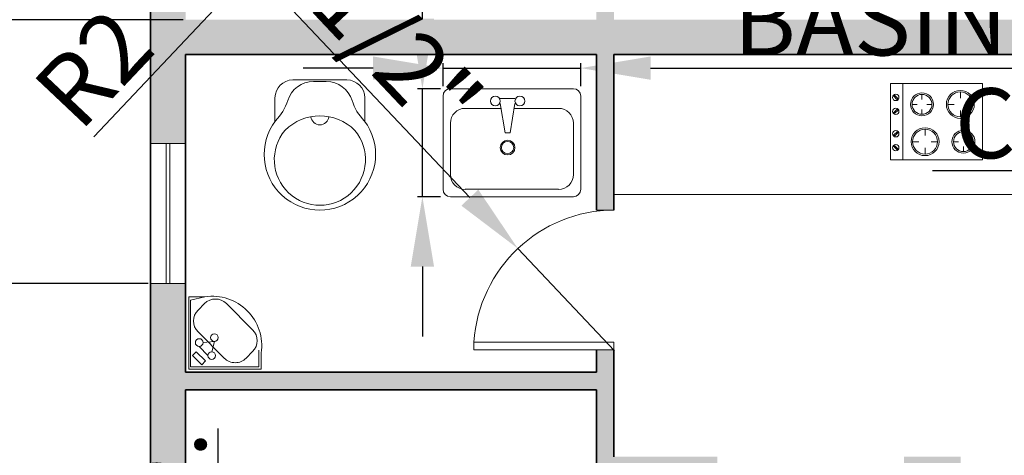
# Model space of a CAD drawing. Units: inches. Extents: x 2043 to 3177, y 1429 to 2563.
# Tile 4 of 14: x 2200 to 2453, y 1840 to 1952. Entities that reach past the tile are written whole.
import ezdxf

# ---------------------------------------------------------------- set-up
doc = ezdxf.new("R2010")
doc.units = ezdxf.units.IN
for name, color, linetype, lineweight in [('A-ANNO-DIMS', 2, 'Continuous', 13), ('A-DOOR', 3, 'Continuous', 18), ('A-EQPM', 8, 'Continuous', 18), ('A-FLOR-CASE', 8, 'Continuous', 18), ('A-FLOR-FIXT', 8, 'Continuous', 18), ('A-GLAZ', 4, 'Continuous', 18), ('A-WALL', 7, 'Continuous', 35)]:
    doc.layers.add(name, color=color, linetype=linetype, lineweight=lineweight)
doc.layers.add('A-WALL-PATT', color=251, linetype='Continuous', lineweight=13, true_color=0x636466)
doc.styles.add('DIM_FONT', font='TXT.shx', dxfattribs={"width": 0.8})
doc.styles.get("Standard").update_dxf_attribs({"font": 'arial.ttf'})
doc.dimstyles.new('ISO-25', dxfattribs={"dimtxt": 18, "dimasz": 18, "dimexe": 1.25, "dimexo": 0.625, "dimtad": 1, "dimlunit": 3, "dimtxsty": 'Standard', "dimcen": 2.5, "dimadec": 0, "dimazin": 0, "dimtfac": 1, "dimtmove": 0, "dimatfit": 3, "dimfxl": 1, "dimarcsym": 0})

# ---------------------------------------------------------------- blocks, each defined once
blk = doc.blocks.new('A$C6EF51710')
at = {"linetype": 'ByBlock'}
for p, q in [((0.0508, 0.2843), (0.1169, 0.2843)), ((0, 0.0811), (0, 0.2335)), ((0.0041, 0.1392), (0.0041, 0.1755)), ((0.1169, 0.0303), (0.0508, 0.0303))]:
    blk.add_line(p, q, dxfattribs=at)
for centre, radius, start, end in [((0.2107, 0.1573), 0.1576, 232.8984, 127.1016), ((0.0508, 0.2335), 0.0508, 90, 180), ((0.0168, 0.3818), 0.1397, 287.1046, 315), ((0.2254, 0.1573), 0.1289, 230.0084, 129.9916), ((0.2413, 0.1573), 0.1397, 135, 225), ((0.0803, 0.1755), 0.0762, 107.1046, 180), ((0.1016, 0.1573), 0.0254, 275.2159, 84.7841), ((0.0803, 0.1392), 0.0762, 180, 252.8954), ((0.0508, 0.0811), 0.0508, 180, 270), ((0.0168, -0.0672), 0.1397, 45, 72.8954)]:
    blk.add_arc(centre, radius, start, end, dxfattribs=at)
blk = doc.blocks.new('A$C03A44EBA')
at = {"rotation": 270}
blk.add_blockref('A$C6EF51710', (0.0003, 0.3683), dxfattribs=at)
blk = doc.blocks.new('A$C564A496C')
at = {"linetype": 'ByBlock'}
for p, q in [((0, 419.3), (0, 30.7)), ((543.2, 450), (30.7, 450)), ((573.8, 30.7), (573.8, 419.3)), ((238.5, 409.1), (299.8, 409.1)), ((238.5, 388.6), (258.9, 265.9)), ((279.4, 265.9), (299.8, 388.6)), ((92, 368.2), (243.6, 368.2)), ((294.7, 368.2), (481.8, 368.2)), ((30.7, 92), (30.7, 306.8)), ((543.2, 306.8), (543.2, 92)), ((258.9, 265.9), (279.4, 265.9)), ((30.7, 0), (543.2, 0)), ((481.8, 30.7), (92, 30.7))]:
    blk.add_line(p, q, dxfattribs=at)
for centre, radius in [((218, 398.9), 20.5), ((320.3, 398.9), 20.5), ((269.1, 204.5), 30.7), ((269.1, 204.5), 25.7)]:
    blk.add_circle(centre, radius, dxfattribs=at)
for centre, radius, start, end in [((30.7, 419.3), 30.7, 90, 180), ((543.2, 419.3), 30.7, 0, 90), ((92, 306.8), 61.4, 90, 180), ((481.8, 306.8), 61.4, 0, 90), ((92, 92), 61.4, 180, 270), ((481.8, 92), 61.4, 270, 0), ((30.7, 30.7), 30.7, 180, 270), ((543.2, 30.7), 30.7, 270, 0)]:
    blk.add_arc(centre, radius, start, end, dxfattribs=at)
at = {"style": 'DIM_FONT', "width": 0.8, "flags": 9}
for tag in ['YSIZE', 'XSIZE']:
    blk.add_attdef(tag, (269.1, 450), '', height=0.5, rotation=270, dxfattribs=at)
blk = doc.blocks.new('A$C017A17F4')
for p, q in [((0.45, 0.45), (0, 0.45)), ((0, 0.45), (0, 0.35)), ((0.45, 0), (0.45, 0.45)), ((0.0533, 0.3414), (0.094, 0.3821)), ((0.2297, 0.3821), (0.3933, 0.2185)), ((0.3467, 0.3997), (0.3704, 0.4234)), ((0.4041, 0.3423), (0.3467, 0.3997)), ((0.3704, 0.4234), (0.4278, 0.366)), ((0.4278, 0.366), (0.4041, 0.3423)), ((0.2168, 0.0421), (0.0533, 0.2056)), ((0.3933, 0.0827), (0.3526, 0.0421)), ((0.35, 0), (0.45, 0))]:
    blk.add_line(p, q)
at = {"ltscale": 10}
for p, q in [((0.4392, 0.4359), (0.0144, 0.4359)), ((0.0144, 0.4359), (0.0144, 0.3323)), ((0.4392, 0.4359), (0.4392, 0.0216)), ((0.3078, 0.342), (0.2911, 0.2778)), ((0.3317, 0.3659), (0.3861, 0.3086)), ((0.3622, 0.2847), (0.2911, 0.2778)), ((0.4392, 0.0216), (0.35, 0))]:
    blk.add_line(p, q, dxfattribs=at)
for centre in [(0.3078, 0.3659), (0.3861, 0.2847), (0.2911, 0.2539)]:
    blk.add_circle(centre, 0.0239, dxfattribs=at)
for centre, radius, start, end in [((0.1618, 0.3142), 0.096, 45, 135), ((0.3045, 0.3045), 0.3079, 171.50989, 278.49011), ((0.1212, 0.2735), 0.096, 135, 225), ((0.3254, 0.1506), 0.096, 315, 45), ((0.2847, 0.11), 0.096, 225, 315)]:
    blk.add_arc(centre, radius, start, end)
blk = doc.blocks.new('*D25')
at = {"layer": 'A-ANNO-DIMS', "color": 0, "lineweight": -2, "transparency": 16777216}
for p, q in [((2233.12, 1884.52), (2167.18, 1884.52)), ((2168.43, 1652.39), (2168.43, 1866.52)), ((2233.12, 1634.39), (2167.18, 1634.39))]:
    blk.add_line(p, q, dxfattribs=at)
at = {"layer": 'A-ANNO-DIMS', "color": 0, "transparency": 16777216}
for points in [[(2165.43, 1866.52), (2171.43, 1866.52), (2168.43, 1884.52)], [(2165.43, 1652.39), (2171.43, 1652.39), (2168.43, 1634.39)]]:
    blk.add_solid(points, dxfattribs=at)
at = {"layer": 'Defpoints', "color": 0, "transparency": 16777216}
for p in [(2168.43, 1884.52), (2233.74, 1884.52), (2233.74, 1634.39)]:
    blk.add_point(p, dxfattribs=at)
at = {"layer": 'A-ANNO-DIMS', "color": 0, "transparency": 16777216, "insert": (2158.61, 1759.46), "char_height": 18, "attachment_point": 5, "rotation": 90}
blk.add_mtext('25\'-0"', dxfattribs=at)
blk = doc.blocks.new('*D26')
at = {"layer": 'A-ANNO-DIMS', "color": 0, "lineweight": -2, "transparency": 16777216}
for p, q in [((2233.12, 2029.27), (2166.79, 2029.27)), ((2168.04, 1902.52), (2168.04, 2011.27)), ((2233.12, 1884.52), (2166.79, 1884.52))]:
    blk.add_line(p, q, dxfattribs=at)
at = {"layer": 'A-ANNO-DIMS', "color": 0, "transparency": 16777216}
for points in [[(2165.04, 2011.27), (2171.04, 2011.27), (2168.04, 2029.27)], [(2165.04, 1902.52), (2171.04, 1902.52), (2168.04, 1884.52)]]:
    blk.add_solid(points, dxfattribs=at)
at = {"layer": 'Defpoints', "color": 0, "transparency": 16777216}
for p in [(2168.04, 2029.27), (2233.74, 2029.27), (2233.74, 1884.52)]:
    blk.add_point(p, dxfattribs=at)
at = {"layer": 'A-ANNO-DIMS', "color": 0, "transparency": 16777216, "insert": (2158.23, 1956.89), "char_height": 18, "attachment_point": 5, "rotation": 90}
blk.add_mtext('19\'-0"', dxfattribs=at)
blk = doc.blocks.new('*D28')
at = {"layer": 'A-ANNO-DIMS', "color": 0, "lineweight": -2, "transparency": 16777216}
for p, q in [((2233.12, 2261.39), (2064.1, 2261.39)), ((2065.35, 2243.39), (2065.35, 1652.39)), ((2233.12, 1634.39), (2064.1, 1634.39))]:
    blk.add_line(p, q, dxfattribs=at)
at = {"layer": 'A-ANNO-DIMS', "color": 0, "transparency": 16777216}
for points in [[(2062.35, 2243.39), (2068.35, 2243.39), (2065.35, 2261.39)], [(2062.35, 1652.39), (2068.35, 1652.39), (2065.35, 1634.39)]]:
    blk.add_solid(points, dxfattribs=at)
at = {"layer": 'Defpoints', "color": 0, "transparency": 16777216}
for p in [(2233.74, 2261.39), (2065.35, 1634.39), (2233.74, 1634.39)]:
    blk.add_point(p, dxfattribs=at)
at = {"layer": 'A-ANNO-DIMS', "color": 0, "transparency": 16777216, "insert": (2055.54, 1947.89), "char_height": 18, "attachment_point": 5, "rotation": 90}
blk.add_mtext('75\'-0"', dxfattribs=at)
blk = doc.blocks.new('A$C16A60262')
at = {"linetype": 'ByBlock'}
for p, q in [((0, 600), (0, 0)), ((487.7, 600), (0, 600)), ((0, 600), (500, 600)), ((0, 600), (500, 600)), ((500, 600), (500, 0)), ((500, 600), (500, 0)), ((500, 520.4), (0, 520.4)), ((119.4, 455.6), (119.4, 414.9)), ((363.3, 459.6), (363.3, 427.1)), ((298.2, 394.6), (330.7, 394.6)), ((428.3, 394.6), (395.8, 394.6)), ((38.1, 374.3), (78.8, 374.3)), ((119.4, 293), (119.4, 333.7)), ((200.7, 374.3), (160.1, 374.3)), ((363.3, 329.6), (363.3, 362.1)), ((363.3, 225.2), (363.3, 184.6)), ((119.4, 188.6), (119.4, 156.1)), ((282, 143.9), (322.6, 143.9)), ((444.5, 143.9), (403.9, 143.9)), ((54.4, 123.6), (86.9, 123.6)), ((119.4, 58.6), (119.4, 91.1)), ((184.4, 123.6), (151.9, 123.6)), ((363.3, 62.6), (363.3, 103.3)), ((0, 0), (500, 0))]:
    blk.add_line(p, q, dxfattribs=at)
for p, q in [((396.2, 558.5), (417.4, 579.7)), ((417.4, 579.7), (423.1, 574)), ((66.2, 557.5), (87.4, 578.7)), ((71.9, 551.8), (66.2, 557.5)), ((93.1, 573), (71.9, 551.8)), ((87.4, 578.7), (93.1, 573)), ((157.6, 572.5), (163.3, 578.1)), ((178.8, 551.2), (157.6, 572.5)), ((163.3, 578.1), (184.5, 556.9)), ((184.5, 556.9), (178.8, 551.2)), ((305.1, 572.5), (310.8, 578.1)), ((326.3, 551.2), (305.1, 572.5)), ((310.8, 578.1), (332, 556.9)), ((332, 556.9), (326.3, 551.2)), ((401.9, 552.8), (396.2, 558.5)), ((423.1, 574), (401.9, 552.8))]:
    blk.add_line(p, q)
for centre in [(80.1, 565.7), (171.2, 565.7), (317.6, 565.7), (408.7, 565.7)]:
    blk.add_circle(centre, 20.6)
for centre, radius in [((119.4, 374.3), 91.3), ((119.4, 374.3), 81.3), ((363.3, 394.6), 75), ((363.3, 394.6), 65), ((119.4, 123.6), 75), ((363.3, 143.9), 91.3), ((363.3, 143.9), 81.3), ((119.4, 123.6), 65)]:
    blk.add_circle(centre, radius, dxfattribs=at)
blk = doc.blocks.new('GLAZING-36')
for p, q in [((0, 36), (0, 0)), ((1, 36), (1, 0))]:
    blk.add_line(p, q)
blk = doc.blocks.new('*D48')
at = {"layer": 'A-ANNO-DIMS', "color": 0, "lineweight": -2, "transparency": 16777216}
for p, q in [((2251.17, 1717.89), (2251.17, 1847.17)), ((2254.14, 1699.89), (2249.92, 1699.89)), ((2251.17, 1675.89), (2251.17, 1699.89)), ((2254.14, 1675.89), (2249.92, 1675.89)), ((2251.17, 1657.89), (2251.17, 1639.89))]:
    blk.add_line(p, q, dxfattribs=at)
at = {"layer": 'A-ANNO-DIMS', "color": 0, "transparency": 16777216}
for points in [[(2248.17, 1717.89), (2254.17, 1717.89), (2251.17, 1699.89)], [(2248.17, 1657.89), (2254.17, 1657.89), (2251.17, 1675.89)]]:
    blk.add_solid(points, dxfattribs=at)
at = {"layer": 'Defpoints', "color": 0, "transparency": 16777216}
for p in [(2251.17, 1699.89), (2254.77, 1699.89), (2254.77, 1675.89)]:
    blk.add_point(p, dxfattribs=at)
at = {"layer": 'A-ANNO-DIMS', "color": 0, "transparency": 16777216, "insert": (2241.35, 1791.53), "char_height": 18, "attachment_point": 5, "rotation": 90}
blk.add_mtext('2\'-0" TYP.', dxfattribs=at)
blk = doc.blocks.new('*D57')
at = {"layer": 'A-ANNO-DIMS', "color": 0, "lineweight": -2, "transparency": 16777216}
for p, q in [((2291.03, 1939.93), (2273.03, 1939.93)), ((2309.03, 1935.24), (2309.03, 1941.18)), ((2309.03, 1939.93), (2344.46, 1939.93)), ((2344.46, 1935.24), (2344.46, 1941.18)), ((2362.46, 1939.93), (2629.01, 1939.93))]:
    blk.add_line(p, q, dxfattribs=at)
at = {"layer": 'A-ANNO-DIMS', "color": 0, "transparency": 16777216}
for points in [[(2291.03, 1942.93), (2291.03, 1936.93), (2309.03, 1939.93)], [(2362.46, 1942.93), (2362.46, 1936.93), (2344.46, 1939.93)]]:
    blk.add_solid(points, dxfattribs=at)
at = {"layer": 'Defpoints', "color": 0, "transparency": 16777216}
for p in [(2344.46, 1939.93), (2309.03, 1934.62), (2344.46, 1934.62)]:
    blk.add_point(p, dxfattribs=at)
at = {"layer": 'A-ANNO-DIMS', "color": 0, "transparency": 16777216, "insert": (2504.74, 1949.86), "char_height": 18, "attachment_point": 5}
blk.add_mtext('BASIN 2\'-11 1/2" TYP.', dxfattribs=at)
blk = doc.blocks.new('*D58')
at = {"layer": 'A-ANNO-DIMS', "color": 0, "lineweight": -2, "transparency": 16777216}
for p, q in [((2303.72, 1952.62), (2303.72, 2081.89)), ((2308.41, 1934.62), (2302.47, 1934.62)), ((2303.72, 1906.83), (2303.72, 1934.62)), ((2308.41, 1906.83), (2302.47, 1906.83)), ((2303.72, 1888.83), (2303.72, 1870.83))]:
    blk.add_line(p, q, dxfattribs=at)
at = {"layer": 'A-ANNO-DIMS', "color": 0, "transparency": 16777216}
for points in [[(2300.72, 1952.62), (2306.72, 1952.62), (2303.72, 1934.62)], [(2300.72, 1888.83), (2306.72, 1888.83), (2303.72, 1906.83)]]:
    blk.add_solid(points, dxfattribs=at)
at = {"layer": 'Defpoints', "color": 0, "transparency": 16777216}
for p in [(2303.72, 1934.62), (2309.03, 1934.62), (2309.03, 1906.83)]:
    blk.add_point(p, dxfattribs=at)
at = {"layer": 'A-ANNO-DIMS', "color": 0, "transparency": 16777216, "insert": (2294.05, 2026.26), "char_height": 18, "attachment_point": 5, "rotation": 90}
blk.add_mtext('2\'-4" TYP.', dxfattribs=at)
blk = doc.blocks.new('*D61')
at = {"layer": 'A-ANNO-DIMS', "color": 0, "lineweight": -2, "transparency": 16777216}
for p, q in [((2770.39, 1916.38), (2770.39, 1912.21)), ((2794.01, 1916.38), (2794.01, 1912.21)), ((2752.39, 1913.46), (2434.98, 1913.46)), ((2794.01, 1913.46), (2770.39, 1913.46)), ((2812.01, 1913.46), (2830.01, 1913.46))]:
    blk.add_line(p, q, dxfattribs=at)
at = {"layer": 'A-ANNO-DIMS', "color": 0, "transparency": 16777216}
for points in [[(2752.39, 1916.46), (2752.39, 1910.46), (2770.39, 1913.46)], [(2812.01, 1916.46), (2812.01, 1910.46), (2794.01, 1913.46)]]:
    blk.add_solid(points, dxfattribs=at)
at = {"layer": 'Defpoints', "color": 0, "transparency": 16777216}
for p in [(2770.39, 1917.01), (2794.01, 1917.01), (2770.39, 1913.46)]:
    blk.add_point(p, dxfattribs=at)
at = {"layer": 'A-ANNO-DIMS', "color": 0, "transparency": 16777216, "insert": (2584.68, 1923.4), "char_height": 18, "attachment_point": 5}
blk.add_mtext('COOKTOP 1\'-11 1/2" TYP.', dxfattribs=at)
blk = doc.blocks.new('*D74')
at = {"layer": 'A-ANNO-DIMS', "color": 0, "lineweight": -2, "transparency": 16777216}
for p, q in [((2242.12, 1952.39), (2178.39, 1952.39)), ((2179.64, 1652.39), (2179.64, 1934.39)), ((2233.12, 1634.39), (2178.39, 1634.39))]:
    blk.add_line(p, q, dxfattribs=at)
at = {"layer": 'A-ANNO-DIMS', "color": 0, "transparency": 16777216}
for points in [[(2176.64, 1934.39), (2182.64, 1934.39), (2179.64, 1952.39)], [(2176.64, 1652.39), (2182.64, 1652.39), (2179.64, 1634.39)]]:
    blk.add_solid(points, dxfattribs=at)
at = {"layer": 'Defpoints', "color": 0, "transparency": 16777216}
for p in [(2179.64, 1952.39), (2242.74, 1952.39), (2233.74, 1634.39)]:
    blk.add_point(p, dxfattribs=at)
at = {"layer": 'A-ANNO-DIMS', "color": 0, "transparency": 16777216, "insert": (2169.83, 1793.39), "char_height": 18, "attachment_point": 5, "rotation": 90}
blk.add_mtext('26\'-6"', dxfattribs=at)
blk = doc.blocks.new('*D86')
at = {"layer": 'A-ANNO-DIMS', "color": 0, "lineweight": -2, "transparency": 16777216}
for p, q in [((2598.87, 1881.94), (2565.26, 1849.73)), ((2451, 1740.24), (2552.26, 1837.28))]:
    blk.add_line(p, q, dxfattribs=at)
at = {"layer": 'A-ANNO-DIMS', "color": 0, "transparency": 16777216}
blk.add_solid([(2550.18, 1839.44), (2554.34, 1835.11), (2565.26, 1849.73)], dxfattribs=at)
at = {"layer": 'Defpoints', "color": 0, "transparency": 16777216}
for p in [(2598.87, 1881.94), (2565.26, 1849.73)]:
    blk.add_point(p, dxfattribs=at)
at = {"layer": 'A-ANNO-DIMS', "color": 0, "transparency": 16777216, "insert": (2488.26, 1789.71), "char_height": 18, "attachment_point": 5, "rotation": 43.781}
blk.add_mtext('R3\'-10 1/2"', dxfattribs=at)
blk = doc.blocks.new('*D91')
at = {"layer": 'A-ANNO-DIMS', "color": 0, "lineweight": -2, "transparency": 16777216}
for p, q in [((2229.24, 1998.38), (2315.93, 1906.58)), ((2353.2, 1867.12), (2328.29, 1893.49))]:
    blk.add_line(p, q, dxfattribs=at)
at = {"layer": 'A-ANNO-DIMS', "color": 0, "transparency": 16777216}
blk.add_solid([(2318.11, 1908.64), (2313.75, 1904.52), (2328.29, 1893.49)], dxfattribs=at)
at = {"layer": 'Defpoints', "color": 0, "transparency": 16777216}
for p in [(2328.29, 1893.49), (2353.2, 1867.12)]:
    blk.add_point(p, dxfattribs=at)
at = {"layer": 'A-ANNO-DIMS', "color": 0, "transparency": 16777216, "insert": (2273.63, 1965.84), "char_height": 18, "attachment_point": 5, "rotation": 313.3628}
blk.add_mtext('R3\'-0 1/2"', dxfattribs=at)
blk = doc.blocks.new('*D92')
at = {"layer": 'A-ANNO-DIMS', "color": 0, "lineweight": -2, "transparency": 16777216}
for p, q in [((2351.56, 2062.42), (2327.82, 2037.29)), ((2219.16, 1922.24), (2315.46, 2024.21))]:
    blk.add_line(p, q, dxfattribs=at)
at = {"layer": 'A-ANNO-DIMS', "color": 0, "transparency": 16777216}
blk.add_solid([(2313.28, 2026.27), (2317.64, 2022.15), (2327.82, 2037.29)], dxfattribs=at)
at = {"layer": 'Defpoints', "color": 0, "transparency": 16777216}
for p in [(2351.56, 2062.42), (2327.82, 2037.29)]:
    blk.add_point(p, dxfattribs=at)
at = {"layer": 'A-ANNO-DIMS', "color": 0, "transparency": 16777216, "insert": (2253.91, 1973.5), "char_height": 18, "attachment_point": 5, "rotation": 46.6358}
blk.add_mtext('R2\'-10 1/2"', dxfattribs=at)

msp = doc.modelspace()

# ---------------------------------------------------------------- hatches: boundary and pattern name
at = {"layer": 'A-WALL-PATT'}
h = msp.add_hatch(color=256, dxfattribs=at)
h.dxf.hatch_style = 1
h.paths.add_polyline_path([(2283.62, 2261.393), (2233.745, 2261.393), (2233.745, 2029.268), (2242.745, 2029.268), (2242.745, 2070.143), (2348.495, 2070.143), (2348.495, 2063.887), (2352.995, 2063.887), (2352.995, 2094.143), (2353.364, 2094.143, -0.017175), (2353.364, 2096.932), (2353.364, 2098.643), (2348.495, 2098.643), (2348.495, 2096.393), (2348.495, 2074.643), (2242.745, 2074.643), (2242.745, 2252.393), (2283.62, 2252.393)])
h.paths.add_polyline_path([(2453.87, 2261.393), (2355.62, 2261.393), (2355.62, 2252.393), (2396.495, 2252.393), (2396.495, 2098.643), (2395.364, 2098.643), (2395.364, 2094.143), (2436.995, 2094.143), (2436.995, 2098.643), (2400.995, 2098.643), (2400.995, 2252.393), (2453.87, 2252.393)])
h.paths.add_polyline_path([(2551.745, 2261.393), (2489.87, 2261.393), (2489.87, 2252.393), (2542.745, 2252.393), (2542.745, 2098.643), (2506.745, 2098.643), (2506.745, 2094.143), (2542.745, 2094.143), (2542.745, 2003.513), (2549.809, 2003.513, -0.0102854), (2551.745, 2003.513), (2551.745, 2195.393), (2571.245, 2195.393), (2571.245, 2204.393), (2551.745, 2204.393)])
h.paths.add_polyline_path([(2724.62, 2261.393), (2662.745, 2261.393), (2662.745, 2204.393), (2643.245, 2204.393), (2643.245, 2195.393), (2662.745, 2195.393), (2662.745, 2002.566, -0.0156152), (2665.651, 2002.566), (2671.745, 2002.566), (2671.745, 2094.143), (2707.745, 2094.143), (2707.745, 2098.643), (2671.745, 2098.643), (2671.745, 2252.393), (2724.62, 2252.393)])
h.paths.add_polyline_path([(2858.87, 2261.393), (2760.62, 2261.393), (2760.62, 2252.393), (2813.495, 2252.393), (2813.495, 2098.643), (2777.495, 2098.643), (2777.495, 2094.143), (2819.302, 2094.143), (2819.302, 2098.643), (2817.995, 2098.643), (2817.995, 2252.393), (2858.87, 2252.393)])
h.paths.add_polyline_path([(2980.745, 2261.393), (2930.87, 2261.393), (2930.87, 2252.393), (2971.745, 2252.393), (2971.745, 2074.643), (2865.995, 2074.643), (2865.995, 2098.643), (2861.429, 2098.643, -0.0279128), (2861.495, 2094.143), (2861.495, 2063.254), (2865.995, 2063.254), (2865.995, 2070.143), (2971.745, 2070.143), (2971.745, 2029.268), (2980.745, 2029.268)])
h.paths.add_polyline_path([(2980.745, 1993.268), (2971.745, 1993.268), (2971.745, 1952.393), (2865.995, 1952.393), (2865.995, 2027.254), (2865.688, 2027.254, -0.0309542), (2861.495, 2027.254), (2861.495, 1952.393), (2671.745, 1952.393), (2671.745, 1954.566), (2662.745, 1954.566), (2662.745, 1883.393), (2661.473, 1883.393, -0.012912), (2661.473, 1880.977), (2661.473, 1874.393), (2671.745, 1874.393), (2671.745, 1943.393), (2861.495, 1943.393), (2861.495, 1903.412, -0.0351753), (2865.995, 1903.659), (2865.995, 1943.393), (2971.745, 1943.393), (2971.745, 1922.018), (2980.745, 1922.018)])
h.paths.add_polyline_path([(2980.745, 1886.018), (2971.745, 1886.018), (2971.745, 1864.643), (2865.995, 1864.643), (2865.995, 1867.412), (2861.495, 1867.412), (2861.495, 1840.643), (2828.844, 1840.643, -0.0159075), (2828.844, 1837.684), (2828.844, 1836.143), (2865.995, 1836.143), (2865.995, 1860.143), (2971.745, 1860.143), (2971.745, 1643.393), (2910.245, 1643.393), (2910.245, 1634.393), (2980.745, 1634.393)])
h.paths.add_polyline_path([(2776.745, 1836.143), (2780.844, 1836.143), (2780.844, 1840.643), (2772.245, 1840.643), (2772.245, 1679.393), (2760.995, 1679.393), (2760.995, 1670.393), (2767.745, 1670.393), (2767.745, 1634.393), (2838.245, 1634.393), (2838.245, 1643.393), (2776.745, 1643.393)])
h.paths.add_polyline_path([(2736.995, 1679.393), (2727.995, 1679.393), (2727.995, 1670.393), (2736.995, 1670.393)])
h.paths.add_polyline_path([(2667.995, 1679.393), (2611.745, 1679.393), (2611.745, 1874.393), (2613.473, 1874.393), (2613.473, 1883.393), (2600.336, 1883.393), (2600.336, 1874.393), (2602.745, 1874.393), (2602.745, 1679.393), (2546.495, 1679.393), (2546.495, 1670.393), (2667.995, 1670.393)])
h.paths.add_polyline_path([(2486.495, 1679.393), (2477.495, 1679.393), (2477.495, 1670.393), (2486.495, 1670.393)])
h.paths.add_polyline_path([(2453.495, 1679.393), (2442.245, 1679.393), (2442.245, 1839.893), (2427.654, 1839.893), (2427.654, 1835.393), (2437.745, 1835.393), (2437.745, 1643.393), (2376.245, 1643.393), (2376.245, 1634.393), (2446.745, 1634.393), (2446.745, 1670.393), (2453.495, 1670.393)])
h.paths.add_polyline_path([(2304.245, 1643.393), (2242.745, 1643.393), (2242.745, 1857.143), (2348.495, 1857.143), (2348.495, 1835.393), (2352.995, 1835.393), (2379.654, 1835.393), (2379.654, 1837.073, -0.0151369), (2379.654, 1839.893), (2352.995, 1839.893), (2352.995, 1867.394), (2348.495, 1867.394), (2348.495, 1861.643), (2242.745, 1861.643), (2242.745, 1884.518), (2233.745, 1884.518), (2233.745, 1634.393), (2304.245, 1634.393)])
h.paths.add_polyline_path([(2551.745, 1955.513), (2542.745, 1955.513), (2542.745, 1952.393), (2352.995, 1952.393), (2352.995, 2027.887, -0.0208198), (2350.117, 2027.887), (2348.495, 2027.887), (2348.495, 1952.393), (2242.745, 1952.393), (2242.745, 1993.268), (2233.745, 1993.268), (2233.745, 1943.393), (2233.745, 1920.518), (2242.745, 1920.518), (2242.745, 1943.393), (2348.495, 1943.393), (2348.495, 1903.394), (2352.995, 1903.394), (2352.995, 1943.393), (2542.745, 1943.393), (2542.745, 1874.393), (2552.336, 1874.393), (2552.336, 1880.494, -0.0155728), (2552.336, 1883.393), (2551.745, 1883.393)])

# ---------------------------------------------------------------- linework, layer by layer
at = {"layer": 'A-DOOR'}
for p, q in [((2348.495, 1903.394), (2352.995, 1903.394)), ((2316.995, 1867.394), (2316.995, 1869.394)), ((2316.995, 1869.394), (2352.995, 1869.394)), ((2352.995, 1869.394), (2352.995, 1867.394)), ((2352.995, 1867.394), (2316.995, 1867.394)), ((2348.495, 1867.394), (2352.995, 1867.394))]:
    msp.add_line(p, q, dxfattribs=at)
msp.add_arc((2353.201, 1867.116), 36.278, 90.3266, 176.40024, dxfattribs=at)
at = {"layer": 'A-FLOR-CASE'}
msp.add_line((2352.995, 1907.393), (2542.745, 1907.393), dxfattribs=at)
at = {"layer": 'A-GLAZ'}
for p, q in [((2242.745, 1920.518), (2233.745, 1920.518)), ((2242.745, 1884.518), (2233.745, 1884.518))]:
    msp.add_line(p, q, dxfattribs=at)
at = {"layer": 'A-WALL'}
for p, q in [((2233.745, 2261.393), (2233.745, 1943.393)), ((2233.745, 1634.393), (2233.745, 1943.393)), ((2242.745, 1943.393), (2348.495, 1943.393)), ((2242.745, 1861.643), (2242.745, 1943.393)), ((2348.495, 1903.394), (2348.495, 1943.393)), ((2352.995, 1943.393), (2542.745, 1943.393)), ((2352.995, 1903.394), (2352.995, 1943.393)), ((2348.495, 1861.643), (2348.495, 1867.394)), ((2352.995, 1839.893), (2352.995, 1867.394)), ((2242.745, 1861.643), (2348.495, 1861.643)), ((2242.745, 1643.393), (2242.745, 1857.143)), ((2242.745, 1857.143), (2348.495, 1857.143)), ((2348.495, 1835.393), (2348.495, 1857.143))]:
    msp.add_line(p, q, dxfattribs=at)

# ---------------------------------------------------------------- block references
at = {"layer": 'A-EQPM', "xscale": 0.0393700787401575, "yscale": 0.0393700787401575, "zscale": 0.0393700787401575, "rotation": 90}
msp.add_blockref('A$C16A60262', (2447.842, 1916.289), dxfattribs=at)
at = {"layer": 'A-FLOR-FIXT'}
for name, p, xscale, yscale, zscale in [('A$C03A44EBA', (2262.989, 1903.362), 91.00031060141868, 91.00031060141868, 91.00031060141868), ('A$C564A496C', (2309.031, 1906.833), 0.0617427035267454, 0.0617427035267454, 0.0617427035267454)]:
    msp.add_blockref(name, p, dxfattribs=dict(at, xscale=xscale, yscale=yscale, zscale=zscale))
at = {"layer": 'A-FLOR-FIXT', "xscale": 41.3428040046008, "yscale": 41.3428040046008, "zscale": 41.3428040046008, "rotation": 180}
msp.add_blockref('A$C017A17F4', (2262.228, 1881.064), dxfattribs=at)
at = {"layer": 'A-GLAZ'}
msp.add_blockref('GLAZING-36', (2237.745, 1884.518), dxfattribs=at)

# ---------------------------------------------------------------- dimensions: what is measured, and where the dimension line sits
at = {"layer": 'A-ANNO-DIMS'}
for base, p1, p2, angle, text, override, picture, middle in [((2065.352, 1634.393), (2233.745, 2261.393), (2233.745, 1634.393), 90, '75\'-0"', {"dimclrd": 0, "dimclre": 0, "dimclrt": 0}, '*D28', (2055.537, 1947.893)), ((2303.717, 1934.617), (2309.031, 1906.833), (2309.031, 1934.617), 90, '<> TYP.', {"dimdec": 1, "dimlfac": 1, "dimrnd": 0, "dimzin": 1, "dimdsep": 46, "dimlunit": 4, "dimfrac": 2}, '*D58', (2294.049, 2026.255)), ((2168.041, 2029.268), (2233.745, 1884.518), (2233.745, 2029.268), 90, '19\'-0"', {"dimclrd": 0, "dimclre": 0, "dimclrt": 0}, '*D26', (2158.225, 1956.893)), ((2770.393, 1913.464), (2794.015, 1917.007), (2770.393, 1917.007), 180, 'COOKTOP <> TYP.', {"dimdec": 1, "dimlfac": 1, "dimrnd": 0, "dimzin": 1, "dimdsep": 46, "dimlunit": 4, "dimfrac": 2}, '*D61', (2584.685, 1923.402)), ((2168.43, 1884.518), (2233.745, 1634.393), (2233.745, 1884.518), 90, '25\'-0"', {"dimclrd": 0, "dimclre": 0, "dimclrt": 0}, '*D25', (2158.615, 1759.456)), ((2251.167, 1699.89), (2254.767, 1675.89), (2254.767, 1699.89), 90, '<> TYP.', {"dimdec": 1, "dimlfac": 1, "dimrnd": 0, "dimzin": 1, "dimdsep": 46, "dimlunit": 4, "dimfrac": 2}, '*D48', (2241.352, 1791.528))]:
    dim = msp.add_linear_dim(base=base, p1=p1, p2=p2, angle=angle, text=text, dimstyle='ISO-25', override=override, dxfattribs=at)
    dim.commit()
    dim.dimension.update_dxf_attribs({"geometry": picture, "text_midpoint": middle})
for center, mpoint, picture, middle in [((2351.556, 2062.422), (2327.822, 2037.293), '*D92', (2253.911, 1973.501)), ((2353.201, 1867.116), (2328.292, 1893.491), '*D91', (2273.63, 1965.844)), ((2598.867, 1881.944), (2565.256, 1849.733), '*D86', (2488.256, 1789.706))]:
    dim = msp.add_radius_dim(center=center, mpoint=mpoint, dimstyle='ISO-25', override={"dimdec": 1, "dimlfac": 1, "dimrnd": 0, "dimzin": 1, "dimdsep": 46, "dimlunit": 4, "dimfrac": 2}, dxfattribs=at)
    dim.commit()
    dim.dimension.update_dxf_attribs({"geometry": picture, "text_midpoint": middle})
dim = msp.add_linear_dim(base=(2344.462, 1939.932), p1=(2309.031, 1934.617), p2=(2344.462, 1934.617), text='BASIN <> TYP.', dimstyle='ISO-25', override={"dimdec": 1, "dimlfac": 1, "dimrnd": 0, "dimzin": 1, "dimdsep": 46, "dimlunit": 4, "dimfrac": 2}, dxfattribs=at)
dim.commit()
dim.dimension.update_dxf_attribs({"geometry": '*D57', "text_midpoint": (2504.735, 1949.864)})
dim = msp.add_linear_dim(base=(2179.645, 1952.393), p1=(2233.745, 1634.393), p2=(2242.745, 1952.393), angle=90, dimstyle='ISO-25', override={"dimdec": 1, "dimlfac": 1, "dimrnd": 0, "dimzin": 1, "dimdsep": 46, "dimlunit": 4, "dimfrac": 2}, dxfattribs=at)
dim.commit()
dim.dimension.update_dxf_attribs({"geometry": '*D74', "text_midpoint": (2169.829, 1793.393)})

doc.saveas('drawing.dxf')
